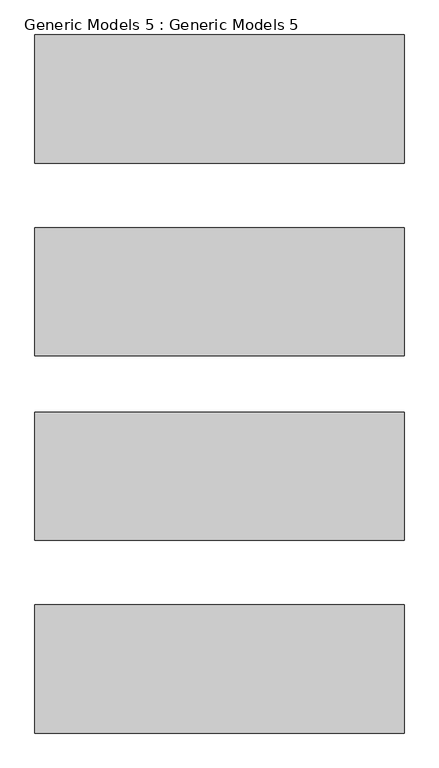
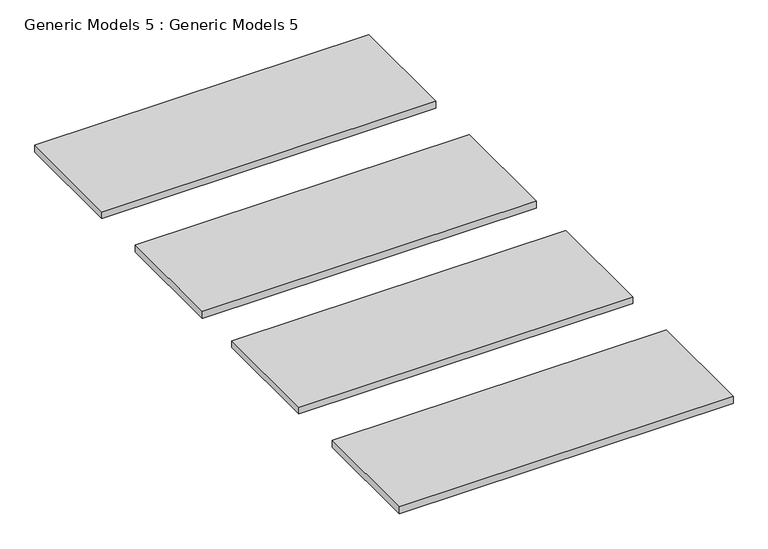
"""IFC4 building model written with IfcOpenShell, lengths in millimetres: proxy geometry, Generic Models 5 : Generic Models 5."""

from ifc_helpers import new_model, si_unit, frame, origin, place, context, project, spatial, polyline, outline, extrude, source, transform, mapped, element, save


def generic_models_5_generic_models_5_6b2521d7(model_context):
    return source(origin(), model_context, "Body", "SweptSolid", [
        extrude(outline(polyline([(-8514.8110257, 1110.4855716), (-8514.8110257, 704.0855716), (-9683.2110257, 704.0855716), (-9683.2110257, 1110.4855716), (-8514.8110257, 1110.4855716)])), frame((0.0, 0.0, -101.6), z_axis=(0.0, 0.0, 1.0), x_axis=(1.0, 0.0, 0.0)), (0.0, 0.0, 1.0), 25.4),
        extrude(outline(polyline([(-8514.8110257, 500.8855716), (-8514.8110257, 94.4855716), (-9683.2110257, 94.4855716), (-9683.2110257, 500.8855716), (-8514.8110257, 500.8855716)])), frame((0.0, 0.0, -101.6), z_axis=(0.0, 0.0, 1.0), x_axis=(1.0, 0.0, 0.0)), (0.0, 0.0, 1.0), 25.4),
        extrude(outline(polyline([(-8514.8110257, -83.3144284), (-8514.8110257, -489.7144284), (-9683.2110257, -489.7144284), (-9683.2110257, -83.3144284), (-8514.8110257, -83.3144284)])), frame((0.0, 0.0, -101.6), z_axis=(0.0, 0.0, 1.0), x_axis=(1.0, 0.0, 0.0)), (0.0, 0.0, 1.0), 25.4),
        extrude(outline(polyline([(-8514.8110257, -692.9144284), (-8514.8110257, -1099.3144284), (-9683.2110257, -1099.3144284), (-9683.2110257, -692.9144284), (-8514.8110257, -692.9144284)])), frame((0.0, 0.0, -101.6), z_axis=(0.0, 0.0, 1.0), x_axis=(1.0, 0.0, 0.0)), (0.0, 0.0, 1.0), 25.4),
    ])


if __name__ == "__main__":
    model = new_model("IFC4")
    model_context = context("Model", 3, world=origin())
    ifc_project = project(units=[si_unit("LENGTHUNIT", "METRE", prefix="MILLI")], contexts=[model_context])
    site = spatial("IfcSite", under=ifc_project)
    building = spatial("IfcBuilding", under=site)
    placement = place(None, origin())
    generic_models_5_generic_models_5_shape = generic_models_5_generic_models_5_6b2521d7(model_context)
    element("IfcBuildingElementProxy", 1, Name="Generic Models 5 : Generic Models 5", ObjectType="Generic Models 5 : Generic Models 5", at=placement, inside=building, context=model_context, shape_type="MappedRepresentation", body=[
        mapped(generic_models_5_generic_models_5_shape, transform((0.0, 0.0, 0.0), x_axis=(1.0, 0.0, 0.0), y_axis=(0.0, 1.0, 0.0), z_axis=(0.0, 0.0, 1.0))),
    ])
    save(model, "model.ifc")

# Revit data of these elements
# Element 1 (IfcBuildingElementProxy, "Generic Models 5 : Generic Models 5")
#   Materials on its faces: "Concrete, Cast-in-Place gray"
# Materials
#   "Concrete, Cast-in-Place gray": class "Concrete", colour RGB 192 192 192, transparency 0, Description = "Cast-in-place concrete", Cost = 0
